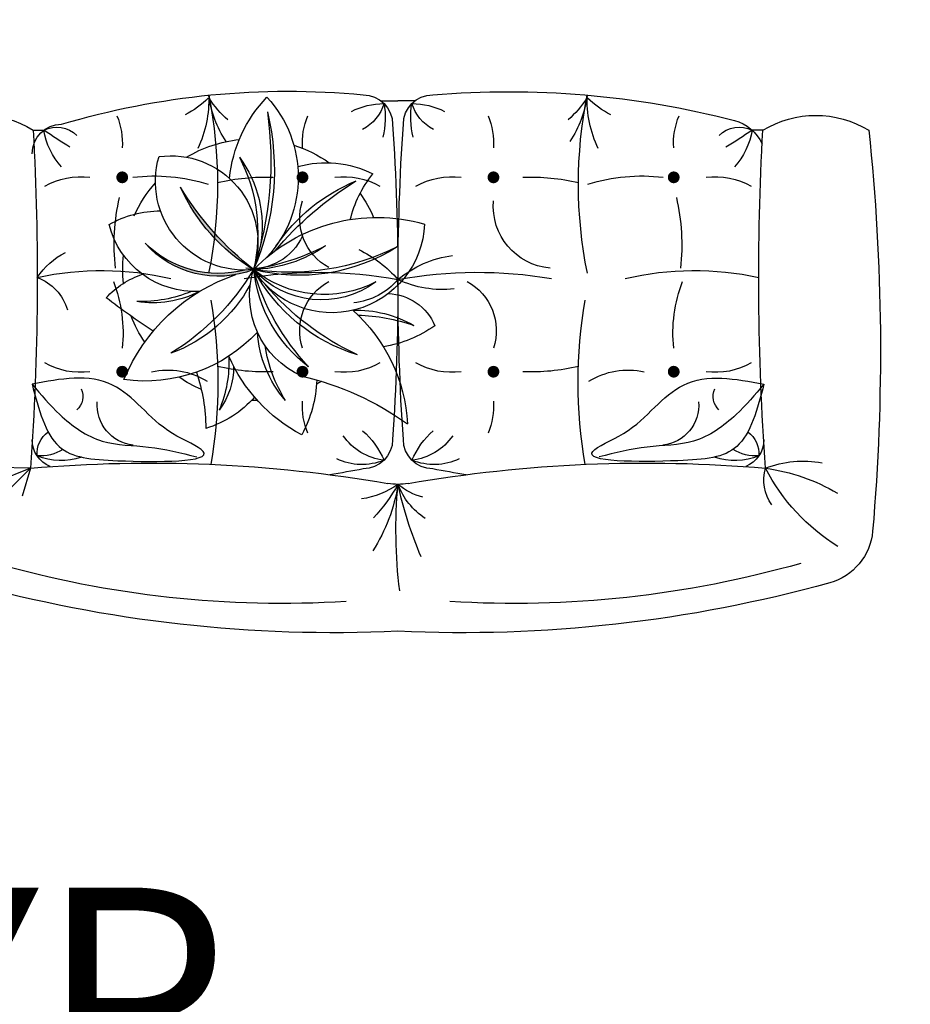
# Model space of a CAD drawing. Units: inches. Extents: x 844 to 2234, y 346 to 1084.
# Tile 5 of 93: x 1112 to 1136, y 653 to 680. Entities that reach past the tile are written whole.
import ezdxf

# ---------------------------------------------------------------- set-up
doc = ezdxf.new("R2010")
doc.units = ezdxf.units.IN
doc.header["$MEASUREMENT"] = 0
doc.layers.add('A-ANNO-DIMS', color=2, linetype='Continuous', lineweight=18)
doc.layers.add('furniture', color=8, linetype='Continuous', lineweight=18)
for name, color, linetype in [('RA-AP-01$0$FURN', 3, 'Continuous'), ('RA-AP-02$0$FLPT', 30, 'Continuous'), ('ROOM-NO', 3, 'Continuous')]:
    doc.layers.add(name, color=color, linetype=linetype)
doc.styles.get("Standard").update_dxf_attribs({"font": 'arial.ttf'})
doc.dimstyles.get("Standard").update_dxf_attribs({"dimtxt": 6, "dimasz": 3, "dimexe": 0.18, "dimexo": 0.0625, "dimgap": 0.09, "dimtad": 0, "dimtih": 1, "dimtoh": 1, "dimdec": 1, "dimzin": 0, "dimdsep": 46, "dimlunit": 3, "dimtxsty": 'Standard', "dimblk": 'ARCHTICK', "dimcen": 0.09, "dimadec": 0, "dimazin": 0, "dimtfac": 1, "dimtdec": 1, "dimtofl": 0, "dimtmove": 0, "dimatfit": 3, "dimfxl": 1, "dimtolj": 1, "dimtzin": 0, "dimarcsym": 0})

# ---------------------------------------------------------------- blocks, each defined once
blk = doc.blocks.new('A$C6E322C05')
at = {"layer": 'RA-AP-01$0$FURN'}
for p, q in [((6.391873508750865, -6.482044957760267), (6.516651486950081, -6.357266979564481)), ((6.391873508750865, -6.482044957760271), (6.43343929223883, -6.37746472106399)), ((6.391873508750866, -6.48204495776027), (6.390422568951521, -6.415535276369585)), ((6.391873508750865, -6.482044957760271), (6.439305270696451, -6.46824831830364)), ((5.817206456966433, -6.486712009544905), (5.817206456965108, -6.505053364959449)), ((5.767206456949363, -7.077520703653457), (5.767206456948565, -7.10671200954539)), ((5.767206456949363, -7.135903315437323), (5.767206456948565, -7.10671200954539)), ((5.817206456966433, -7.726712009545875), (5.817206456965108, -7.70837065413133))]:
    blk.add_line(p, q, dxfattribs=at)
at = {"layer": 'RA-AP-01$0$FURN', "const_width": 0.01}
for points in [[(5.902459393885763, -6.638129816788149, 1), (5.892459393885761, -6.638129816788122, 1)], [(6.222844373610339, -6.638129816788595, -1), (6.23284437361034, -6.638129816788595, -1)], [(5.902459393885763, -6.944444251846759, -1), (5.892459393885761, -6.944444251846785, -1)], [(6.222844373610339, -6.944444251846313, 1), (6.23284437361034, -6.944444251846313, 1)], [(5.902459393885763, -7.268979767244021, 1), (5.892459393885761, -7.268979767243994, 1)], [(6.222844373610339, -7.268979767244466, -1), (6.23284437361034, -7.268979767244466, -1)], [(5.902459393885763, -7.575294202302631, -1), (5.892459393885761, -7.575294202302657, -1)], [(6.222844373610339, -7.575294202302185, 1), (6.23284437361034, -7.575294202302185, 1)]]:
    blk.add_lwpolyline(points, format="xyb", close=True, dxfattribs=at)
at = {"layer": 'RA-AP-01$0$FURN'}
for centre, radius, start, end in [((6.192206456970573, -9.839674509409203), 3.552808610866049, 85.0473312316412, 96.0588723756579), ((5.962206456956505, -6.396712009545393), 0.1706604816468166, 148.1725534208377, 211.8274465791593), ((6.490296991311982, -6.399757455669855), 0.1, 15.49949460085664, 85.04733123164101), ((4.33669785707999, -6.99698289606033), 2.33487526667919, 357.3063521928599, 15.49949460085664), ((4.846593614069285, -6.909687157115225), 1.775196618325768, 356.4780136403396, 15.93354743557553), ((5.857266904022845, -6.534972599266733), 0.05, 90.00000000094654, 180), ((6.068281987477935, -2.019830784287151), 4.473931917517753, 266.7828902523826, 274.1477233631118), ((6.367926665937501, -6.54114871013533), 0.0478550828899777, 86.575295631534, 142.6833829238214), ((6.343036863464309, -6.534972599266733), 0.05, 22.58267242460392, 89.99999999905346), ((6.302747869360707, -6.499593011892033), 0.0683206773889159, 326.6729861493449, 5.218395042636973), ((6.274768375315671, -6.53387763124781), 0.1042084262671507, 340.4828318717155, 22.86929393278168), ((8.747044799885572, -6.68548500417652), 2.363941552380466, 175.0630368065897, 189.8434409139549), ((5.860011614985668, -6.526983908613928), 0.0479292786975047, 152.8070868543555, 225.4025460716553), ((5.798239671935704, -6.625433523557484), 0.1218651776285568, 48.0375529564433, 81.0462320954125), ((4.904259194880517, -7.136565421857206), 1.11020813118073, 31.93286085977143, 34.66647731879807), ((6.017778833798976, -6.566879816788349), 0.1214118203512435, 150.1419074485596, 187.691663289156), ((6.134026645419561, -6.595486433826224), 0.1214600988114338, 123.1053299945123, 153.7006015369794), ((6.565877894706778, -6.603111116245941), 0.5100538472773755, 167.6182489359307, 193.3122231353938), ((6.14746341585187, -6.463466129962243), 0.0853281020358404, 200.7831020638199, 253.0462459140071), ((6.107524933697323, -6.566879816788473), 0.1214118203512435, 352.3083367106845, 29.85809255128089), ((7.09459581372041, -6.919286936999045), 1.343470592134322, 163.3777289595395, 185.4806594039327), ((6.269780256940199, -6.54020363968894), 0.0310151388417235, 245.7760318513891, 317.3789451550392), ((6.284290296802319, -6.664490968717984), 0.0689028341546707, 6.419517109091462, 94.46157264568865), ((6.011601695098697, -6.976164478788355), 0.3517162425384579, 83.41248966761121, 103.1674570565571), ((6.162348040003244, -6.395238182300004), 0.2442261434243043, 248.9017070735605, 275.9923925191661), ((5.839565409091811, -6.517091257029312), 0.1212957045587361, 247.3375839744822, 273.7314750942433), ((6.197523316847625, -6.692545952238853), 0.3023568492824586, 173.0944825511667, 197.588060785551), ((6.354517986346992, -6.715077923337803), 0.1295083186917369, 167.9901339202812, 211.3796151021958), ((5.650260521516567, -6.673548227893377), 0.1579426672576338, 315.4052081938554, 333.0844958846701), ((5.765922189292775, -6.593612516654137), 0.1915923630277471, 267.5852697713958, 295.5830728418392), ((5.908792452070163, -6.03459657477793), 0.765467899454341, 258.6273206109321, 281.4174148186357), ((5.73314461686815, -6.969744817001631), 0.1863549309199891, 56.29262493376822, 82.3818003344588), ((5.679375702373212, -6.920075501166131), 0.1579426672576338, 40.38651175517922, 58.06579944599388), ((6.245858341704271, -5.977214432993086), 0.8232838708255751, 260.2449188973366, 279.7550811026635), ((6.245792934290092, -6.879444251846194), 0.3486563571350461, 166.839178360846, 182.4657575311016), ((5.879510833205829, -6.879444251846704), 0.3486563571350461, 357.5342424690579, 13.1608216393135), ((5.959527339947079, -6.859074294904489), 0.0930420630931112, 293.6025128512426, 6.610683813350465), ((6.80739198570858, -6.9716011229856), 0.7485435294774117, 170.3094183042209, 190.3986311369044), ((5.839565409091811, -7.065482811605596), 0.1212957045587361, 86.2685249057567, 112.6624160255178), ((5.967289987028921, -7.035039638983766), 0.0953802309589454, 28.80342840007747, 108.2253060204472), ((6.158013780467433, -7.035039638983501), 0.0953802309589454, 71.7746939797123, 151.196571600082), ((6.285738358404627, -7.065482811604976), 0.1212957045587361, 67.33758397464167, 93.73147509440282), ((5.08702348459791, -6.791287034316994), 1.330927509443381, 348.8964178164725, 351.3771209523497), ((6.017778833798976, -7.015694251846559), 0.1214118203512435, 172.308336710844, 209.8580925514404), ((6.107524933697323, -7.015694251846435), 0.1214118203512435, 330.1419074487191, 7.691663289315497), ((6.286338558013386, -7.045586518350251), 0.0993499474027353, 337.9047121936679, 25.63436525513283), ((5.904234274973987, -7.085727051545815), 0.1323517050571434, 153.8887786398558, 178.8006589660143), ((6.280014948979332, -7.094901076442985), 0.0990996950214925, 6.922564260119504, 55.10883789097723), ((6.211136556040091, -6.947122539501678), 0.212288550941915, 205.9704430982785, 228.7419974602242), ((5.999456242224805, -7.021102361717039), 0.1116589361851176, 309.9425663137084, 354.6905921774272), ((6.304557655687245, -7.024767404076127), 0.1410608784479501, 324.4849629611242, 351.797284145529), ((5.807266904022846, -7.047601469367252), 0.05, 180, 269.9999999990534), ((5.751472800077547, -7.013313769593298), 0.07258027258109, 286.3558526771587, 332.6774804096085), ((6.4323439288987, -6.955317466880212), 0.1385734111998875, 221.2288777133949, 247.0867614897648), ((6.343036863466045, -7.047601469376512), 0.05, 269.9999999989608, 359.9999999989431), ((6.374625390672053, -6.818147225624045), 0.2920141296149301, 278.8152064253152, 302.6921045175205), ((6.285596300104752, -6.865193601455727), 0.2760944594998999, 298.9825510110601, 313.6694461006315), ((5.795585623761384, -6.952739633017071), 0.1323517050571434, 259.6959164764198, 284.6077968025783), ((6.319376003798462, -7.10671200954539), 0.1, 350.1565590860452, 9.843440913955273), ((6.075151883811576, -3.163731520221818), 3.942980489323571, 266.1043400737264, 273.8956599242929), ((6.075151883808545, -11.04969249895812), 3.942980489412734, 86.10434007575122, 93.89565992614118), ((6.213892115887508, -7.225151532818968), 0.1854874288882049, 140.3167953258794, 172.0522897837384), ((6.80739198570858, -7.241822896105179), 0.7485435294774117, 169.6010516837189, 189.690581695779), ((5.911254573522987, -7.182496879996349), 0.1769409696162427, 353.679636560008, 25.3608296845614), ((6.496371549498975, -7.961935855380467), 0.8586827939016008, 83.03755924582121, 95.14445252709366), ((6.375720249476352, -7.220682794696101), 0.1220457486080966, 33.71356548940426, 69.04099283815023), ((6.338324584842819, -7.175279287582296), 0.1061640434993627, 14.36483859718907, 40.23030537468725), ((6.269502792941208, -7.789055933740261), 0.6986094833441214, 67.00911261779231, 77.61200156369726), ((4.336697857080025, -7.216441123030454), 2.334875266679154, 344.5005053991432, 2.69364780714023), ((5.807266904022846, -7.165822549723527), 0.05, 90.00000000094654, 180), ((5.795585623761384, -7.260684386073708), 0.1323517050571434, 75.39220319742172, 100.3040835235802), ((6.343036863466045, -7.165822549714267), 0.05, 1.0568602e-09, 90.00000000103913), ((8.747044799885572, -7.527939014914259), 2.363941552380466, 170.156559086045, 184.9369631934102), ((5.904234274973987, -7.127696967544965), 0.1323517050571434, 181.1993410339857, 206.1112213601442), ((5.751472800077547, -7.200110249497481), 0.07258027258109, 27.32251959039153, 73.64414732284132), ((6.017778833798976, -7.19772976724422), 0.1214118203512435, 150.1419074485596, 187.691663289156), ((6.107524933697323, -7.197729767244345), 0.1214118203512435, 352.3083367106845, 29.85809255128088), ((6.4323439288987, -7.25810655221026), 0.1385734111998875, 112.9132385102352, 138.7711222866051), ((6.280014948979332, -7.118522942647487), 0.0990996950214925, 304.8911621090228, 353.0774357398805), ((6.286338558013386, -7.167837500740221), 0.0993499474027353, 334.3656347448672, 22.09528780633203), ((7.290981934450236, -7.293982589837588), 1.539060359583382, 175.2233567466078, 194.4661216781742), ((5.08702348459791, -7.422136984773786), 1.330927509443381, 8.62287904765033, 11.10358218352746), ((4.846593614069285, -7.303736861975558), 1.775196618325768, 344.0664525644245, 3.521986359660393), ((6.158013780467433, -7.178384380107278), 0.0953802309589454, 208.803428399918, 288.2253060202877), ((5.839565409091811, -7.147941207485184), 0.1212957045587361, 247.3375839744822, 273.7314750942433), ((6.285738358404627, -7.147941207485803), 0.1212957045587361, 266.2685249055972, 292.6624160253583), ((5.946346035540796, -7.374645549675604), 0.1060388135390937, 5.185910074000148, 94.80734315124221), ((6.245792934290092, -7.333979767244585), 0.3486563571350461, 177.5342424688983, 193.160821639154), ((5.879510833205829, -7.333979767244075), 0.3486563571350461, 346.8391783606865, 2.465757530942165), ((5.679375702373212, -7.293348517924648), 0.1579426672576338, 301.9342005540061, 319.6134882448208), ((5.73314461686815, -7.243679202089149), 0.1863549309199891, 277.6181996655412, 303.7073750662318), ((5.908792452070163, -8.17882744431285), 0.765467899454341, 78.58258518136427, 101.3726793890678), ((6.245858341704271, -8.236209586097694), 0.8232838708255751, 80.24491889733653, 99.75508110266345), ((5.765922189292775, -7.619811502436642), 0.1915923630277471, 64.41692715816083, 92.41473022860427), ((5.650260521516567, -7.539875791197403), 0.1579426672576338, 26.91550411532996, 44.59479180614462), ((6.197523316847625, -7.520878066851927), 0.3023568492824586, 162.411939214449, 186.9055174488332), ((6.354517986346992, -7.498346095752976), 0.1295083186917369, 148.6203848978042, 192.0098660797188), ((6.565877894706778, -7.610312902844838), 0.5100538472773755, 166.6877768646062, 192.3817510640693), ((6.284290296802319, -7.548933050372795), 0.0689028341546707, 265.5384273543114, 353.5804828909086), ((5.839565409091811, -7.696332762061468), 0.1212957045587361, 86.26852490575668, 112.6624160255178), ((6.011601695098697, -7.237259540302424), 0.3517162425384579, 256.8325429434429, 276.5875103323888), ((6.162348040003244, -7.818185836790775), 0.2442261434243043, 84.00760748083387, 111.0982929264395), ((6.017778833798976, -7.646544202302431), 0.1214118203512435, 172.308336710844, 209.8580925514404), ((6.107524933697323, -7.646544202302306), 0.1214118203512435, 330.1419074487191, 7.691663289315504), ((6.269780256940199, -7.67322037940184), 0.0310151388417235, 42.62105484496073, 114.2239681486109), ((6.274768375315671, -7.679546387842969), 0.1042084262671507, 337.1307060672183, 19.51716812828453), ((5.860011614985668, -7.686440110476851), 0.0479292786975047, 134.5974539283447, 207.1929131456445), ((4.904259194880517, -7.076858597233573), 1.11020813118073, 325.333522681202, 328.0671391402286), ((5.87316911435942, -7.657653239374848), 0.0753785023123622, 196.0166452769965, 244.1254380939442), ((5.798239671935704, -7.587990495533295), 0.1218651776285568, 278.9537679045876, 311.9624470435567), ((6.302747869360707, -7.713831007198747), 0.0683206773889159, 354.781604957363, 33.32701385065516), ((6.343036863464309, -7.678451419824046), 0.05, 270.0000000009465, 337.4173275753961), ((6.367926665937501, -7.672275308955449), 0.0478550828899777, 217.3166170761785, 273.424704368466), ((5.966706456956126, -7.816712009545387), 0.1744999999876311, 148.9517780040469, 211.0482219959533), ((6.068281987477935, -12.19359323480363), 4.473931917517753, 85.85227663688822, 93.21710974761734), ((6.549562589740832, -7.794613830093475), 0.1698955038956699, 158.1487616198804, 191.122156864055), ((6.412319729336772, -7.798818772412041), 0.0704710051510922, 53.58735038429053, 106.8661365794674), ((6.713110001951175, -7.687961227420911), 0.3241573581843151, 187.6973649013944, 210.7014325157311), ((6.237117433414106, -8.032110101276656), 0.3382138395168437, 31.74362916573515, 62.76966729059727), ((6.49029699131198, -7.813666563420925), 0.1, 274.9526687683584, 344.500505399143), ((6.192206456970577, -4.373749509681577), 3.552808610866049, 263.941127624342, 274.9526687683587)]:
    blk.add_arc(centre, radius, start, end, dxfattribs=at)
for points, knots in [([(6.249068123947751, -6.484897777661085), (6.239897409094627, -6.533353418276971), (6.226611264288107, -6.603553906267942), (6.290696373977354, -6.673990528916563), (6.332121563214334, -6.713363084361603), (6.381789098403072, -6.831232979612737), (6.381738454094183, -6.629656072516828), (6.370771929626907, -6.516634365426866), (6.291185937762818, -6.495880800642047), (6.249068123947751, -6.484897777661087)], [0, 0, 0, 0, 0.1367586589314792, 0.1981301758052368, 0.2677729570689282, 0.3281194902553322, 0.4737578340741565, 0.5765194025309516, 0.6920332287422236, 0.6920332287422236, 0.6920332287422236, 0.6920332287422236]), ([(6.249068123947751, -6.484897777661087), (6.266851662635476, -6.499857019491296), (6.306238891621481, -6.532988956490432), (6.353826300430336, -6.600137645661404), (6.352465874908733, -6.685122080531377), (6.365878290565239, -6.737689715716581), (6.372748706337224, -6.764617117843226)], [0, 0, 0, 0, 0.070018540671015, 0.1550780383534498, 0.2344491945777043, 0.3178048737568289, 0.3178048737568289, 0.3178048737568289, 0.3178048737568289]), ([(6.249068123947751, -7.728526241429694), (6.239897409094627, -7.680070600813808), (6.226611264288107, -7.609870112822835), (6.290696373977354, -7.539433490174218), (6.332121563214334, -7.500060934729178), (6.381789098403072, -7.382191039478041), (6.381738454094183, -7.583767946573952), (6.370771929626907, -7.696789653663914), (6.291185937762818, -7.717543218448732), (6.249068123947751, -7.728526241429692)], [0, 0, 0, 0, 0.1367586589314792, 0.1981301758052368, 0.2677729570689282, 0.3281194902553322, 0.4737578340741565, 0.5765194025309516, 0.6920332287422236, 0.6920332287422236, 0.6920332287422236, 0.6920332287422236]), ([(6.249068123947751, -7.728526241429692), (6.266851662635476, -7.713566999599485), (6.306238891621481, -7.680435062600349), (6.353826300430336, -7.613286373429378), (6.352465874908733, -7.528301938559401), (6.365878290565239, -7.475734303374198), (6.372748706337224, -7.448806901247554)], [0, 0, 0, 0, 0.070018540671015, 0.1550780383534498, 0.2344491945777043, 0.3178048737568289, 0.3178048737568289, 0.3178048737568289, 0.3178048737568289])]:
    blk.add_open_spline(points, degree=3, knots=knots, dxfattribs=at)
blk = doc.blocks.new('A$C78016F37')
at = {"layer": 'RA-AP-02$0$FLPT'}
for points in [[(8.585816203069419, -6.02390819987247, -0.263770389754008), (8.460672408962632, -5.900531828839305, -0.0241291823863587), (8.454072418949808, -5.887595694471202, 2.53684562776e-05), (8.45404743172537, -5.887630207283394, 0.3135010205465867)], [(8.6375288720004, -5.923949758415821, -0.0887687358956854), (8.454121692088984, -5.887527659105068, 7.7903089823e-06), (8.45411401635844, -5.887538255716633, 0.1521261679004899)]]:
    blk.add_hatch(color=256, dxfattribs=at).paths.add_polyline_path(points)
at = {"layer": 'RA-AP-01$0$FURN'}
for centre, radius, start, end in [((8.676215054199671, -5.667660989702041), 0.3125591380039201, 178.1117989109854, 224.6938723266582), ((8.77416640415315, -5.62926868308301), 0.4113013577889528, 183.916601998098, 218.889069239545), ((8.454024671827373, -5.887489670112504), 0.2224048992971994, 84.85146405771819, 96.8968759960221), ((7.926806489084671, -5.648344237112944), 0.5693232143741963, 340.3683676450975, 358.6332230039188), ((8.195746570571197, -5.703566525505195), 0.3030929277970076, 334.410018118324, 8.056842366720524), ((8.454024671827373, -5.887489670112504), 0.2224048992971994, 48.29632106119188, 65.66234443375417), ((8.028579057188336, -5.942548842808446), 0.3176725093823991, 32.12276904396682, 49.65676958807643), ((8.138392155386812, -5.868774225710474), 0.1937166188785145, 28.24647600965292, 60.3482035660113), ((8.485489110864293, -5.735116799889917), 0.1555876039528135, 173.9896977683083, 258.3326220930856), ((8.521327457039675, -5.708924385009453), 0.1908277389198635, 182.9741757068071, 249.3481441545862), ((8.654249619708994, -5.778555799161595), 0.2279399438329033, 175.7401143551485, 208.5487298435666), ((8.841321835932057, -5.738299260526738), 0.4150383977849519, 183.2217031044116, 201.067141094303), ((8.454024671827373, -5.887489670112504), 0.2224048992971994, 359.5998786150253, 24.14255533511359), ((8.442163868805496, -5.589503946884691), 0.2981456377964393, 227.2393731923049, 272.0875214538299), ((8.499731284894388, -5.433816546692462), 0.4559697329776795, 235.2365058162176, 260.2774785796924), ((8.645911592327788, -6.090477518425219), 0.27932894017942, 93.04938662579335, 133.3896949469156), ((8.610008543493892, -6.006599373458567), 0.1961871509349957, 83.84242350983102, 130.6121505715144), ((8.564547574985227, -5.985184712735347), 0.1475114689626245, 22.41040215178937, 138.5254141817128), ((8.454024671827373, -5.887489670112504), 0.2224048992971994, 179.1222698891959, 181.6416201752811), ((8.343226438185093, -5.786283478281637), 0.1500631261941314, 234.481997856841, 317.590554229248), ((8.35533458686642, -5.671200371653297), 0.2372928460263133, 247.4602721701189, 294.3106346998744), ((8.353310301606033, -5.50080131865886), 0.3995888706145134, 257.1400840392136, 284.5985568218482), ((8.820839898988444, -6.089372712149781), 0.4186128907603021, 151.1845644972185, 178.7925181665867), ((8.647592804319403, -5.39327801538501), 0.5307671632505924, 248.6111860886518, 268.9135435570199), ((8.591324349397098, -5.825721750746069), 0.1505539017216363, 204.2218678925879, 316.713948440902), ((8.60427433017431, -5.61130057980146), 0.3144127437625546, 241.4533621372112, 276.0713675084609), ((8.617925276426345, -5.861018191689067), 0.1660245384207697, 189.1745772070899, 258.8487542743241), ((8.650970463531563, -6.036034461900849), 0.252604074752176, 148.7548044074418, 190.1503402437527), ((8.632043935228618, -5.851861780578565), 0.1781487401371014, 195.8547118906642, 254.9602254039967), ((8.27103219642381, -5.762377687346963), 0.1942058542978326, 259.1738264472347, 296.9361074578899), ((8.242487148295718, -5.713440208635033), 0.2398180026482373, 268.1044384936476, 291.9165885710061), ((8.454024671827373, -5.887489670112504), 0.2224048992971994, 324.5751954876287, 341.8360454133948), ((8.643418645519843, -5.97565241718072), 0.1753165964770544, 183.2000241261284, 219.1319783506275), ((8.454024671827373, -5.887489670112504), 0.2224048992971994, 208.6999597596628, 211.2898901048327), ((8.447576280134497, -6.186493140077375), 0.2128537218708566, 117.7922244992203, 143.1680179163233), ((8.391080266506174, -6.106601067273632), 0.1233275614230441, 120.0065551025349, 157.0200898875673), ((8.702436309821351, -5.965526387054176), 0.2293777808440535, 187.970132899875, 211.770006950379), ((8.454024671827373, -5.887489670112504), 0.2224048992971994, 233.8814212202215, 245.0364073377333), ((8.454024671827373, -5.887489670112504), 0.2224048992971994, 294.3332330132876, 306.7022905924929), ((8.454024671827373, -5.887489670112504), 0.2224048992971994, 266.6746775461067, 279.4836973606225)]:
    blk.add_arc(centre, radius, start, end, dxfattribs=at)
at = {"layer": 'RA-AP-02$0$FLPT'}
blk.add_lwpolyline([(8.373681407360612, -5.597603282219753, 0.7334826821515817), (8.454024671827373, -5.887489670112506, 0.2766279680881699), (8.373681407360612, -5.597603282219752, 1.3559471233864)], format="xyb", dxfattribs=at)
for centre, radius, start, end in [((8.307234168263015, -5.560224752275053), 0.1974581866646199, 313.6950443365965, 339.1517930721081), ((8.39717548070647, -5.778250590985688), 0.1754354389711152, 14.56900959352841, 57.37320031926483), ((8.423880035729836, -5.687934118592295), 0.2086915776254087, 175.0742803806306, 201.2122531761669), ((8.228139151249446, -5.75774524127399), 0.0885717136803359, 32.28640253436571, 97.90409188948885), ((8.433135668112254, -6.051756800567661), 0.1760533926534347, 161.4400574260173, 193.8427700955681), ((8.395985399479063, -6.084837299933293), 0.1497734353479364, 343.3485825573843, 11.74756506179821), ((8.41746442128814, -6.364284642428606), 0.3118134108627832, 101.9980156162763, 119.8647524560376), ((8.942045887600607, -5.120169675385827), 1.085029101271162, 243.0359441902965, 248.2214525024466)]:
    blk.add_arc(centre, radius, start, end, dxfattribs=at)
at = {"layer": 'ROOM-NO'}
for centre, radius, start, end in [((8.65235909715731, -5.915275987506324), 0.2002713751519826, 77.61332513631854, 163.1649854687259), ((8.46944987509335, -5.65497750757116), 0.2349499976215632, 306.2836330402241, 344.0182681768919), ((8.897731643814414, -6.279909663508004), 0.5923422390868573, 112.2662452820337, 138.5100534847894), ((8.794175340646271, -6.133856003178959), 0.4198977696908007, 106.7322927724504, 144.0984247900076), ((8.22288024947718, -6.040653787747125), 0.2772850355038946, 71.89678357893693, 117.3860017964977), ((7.898132843717886, -6.242790504972724), 0.48979813475044, 43.05187184217114, 66.25811984072557), ((8.347851773195234, -6.064576052783105), 0.2064758371609359, 122.2147792747386, 149.2270256684313), ((8.154124515379644, -5.981454547332234), 0.314276155615234, 322.6594768637323, 11.71644421186061), ((8.609526443069848, -6.010438452646774), 0.261483616160276, 163.3494523104177, 218.1824089018609), ((8.3154997513214, -5.724318991124441), 0.2758350084868725, 238.2734303421065, 276.8355613505966), ((8.468611314717652, -6.062483436674201), 0.1756006505860901, 0.6277371554985871, 30.43990742705027), ((8.602078464955955, -5.915823919619132), 0.1507406891149966, 207.5045866236536, 286.2267783265413)]:
    blk.add_arc(centre, radius, start, end, dxfattribs=at)
blk = doc.blocks.new('A$C5D2F253E')
at = {"layer": 'RA-AP-01$0$FURN', "xscale": -1}
blk.add_blockref('A$C6E322C05', (4.620200485489021, 7.961130550668883), dxfattribs=at)
at = {"layer": 'RA-AP-02$0$FLPT', "xscale": -1, "rotation": 210.3787734063952}
blk.add_blockref('A$C78016F37', (-5.749960471669055, -8.254610923396115), dxfattribs=at)
blk = doc.blocks.new('_ArchTick')
at = {"color": 0, "linetype": 'ByBlock', "const_width": 0.15}
blk.add_lwpolyline([(-0.5, -0.5), (0.5, 0.5)], dxfattribs=at)
blk = doc.blocks.new('*D107')
at = {"layer": 'A-ANNO-DIMS', "color": 0, "lineweight": -2, "transparency": 16777216}
for p, q in [((983.441711364941, 646.5161314192717), (983.441711364941, 653.8336314192717)), ((983.441711364941, 653.6536314192717), (1031.441711364941, 653.6536314192717)), ((1031.441711364941, 646.5161314192717), (1031.441711364941, 653.8336314192717)), ((1031.441711364941, 653.6536314192717), (1034.441711364941, 653.6536314192717))]:
    blk.add_line(p, q, dxfattribs=at)
at = {"layer": 'Defpoints', "color": 0, "transparency": 16777216}
for p in [(1031.441711364941, 653.6536314192717), (983.441711364941, 646.4536314192717), (1031.441711364941, 646.4536314192717)]:
    blk.add_point(p, dxfattribs=at)
at = {"layer": 'A-ANNO-DIMS', "color": 0, "lineweight": -2, "transparency": 16777216, "xscale": 3, "yscale": 3, "zscale": 3, "rotation": 180}
blk.add_blockref('_ArchTick', (983.441711364941, 653.6536314192717), dxfattribs=at)
at = {"layer": 'A-ANNO-DIMS', "color": 0, "lineweight": -2, "transparency": 16777216, "xscale": 3, "yscale": 3, "zscale": 3}
blk.add_blockref('_ArchTick', (1031.441711364941, 653.6536314192717), dxfattribs=at)
at = {"layer": 'A-ANNO-DIMS', "color": 0, "transparency": 16777216, "insert": (1078.786827326742, 653.6536314192717), "char_height": 6, "attachment_point": 5}
blk.add_mtext('\\A1;WARDROBE 4\'-0" TYP.', dxfattribs=at)
blk = doc.blocks.new('*D144')
at = {"layer": 'A-ANNO-DIMS', "color": 0, "lineweight": -2, "transparency": 16777216}
for p, q in [((1096.615948, 439.3732739999999), (1096.615948, 1074.743301)), ((1143.115948, 492.373274), (1143.115948, 1074.743301)), ((1096.615948, 1074.563301), (1102.481950728513, 1074.563301)), ((1143.115948, 1074.563301), (1137.249945271487, 1074.563301))]:
    blk.add_line(p, q, dxfattribs=at)
at = {"layer": 'Defpoints', "color": 0, "transparency": 16777216}
for p in [(1143.115948, 1074.563301), (1143.115948, 492.3107739999999), (1096.615948, 439.3107739999999)]:
    blk.add_point(p, dxfattribs=at)
at = {"layer": 'A-ANNO-DIMS', "color": 0, "lineweight": -2, "transparency": 16777216, "xscale": 3, "yscale": 3, "zscale": 3, "rotation": 180}
blk.add_blockref('_ArchTick', (1096.615948, 1074.563301), dxfattribs=at)
at = {"layer": 'A-ANNO-DIMS', "color": 0, "lineweight": -2, "transparency": 16777216, "xscale": 3, "yscale": 3, "zscale": 3}
blk.add_blockref('_ArchTick', (1143.115948, 1074.563301), dxfattribs=at)
at = {"layer": 'A-ANNO-DIMS', "color": 0, "transparency": 16777216, "insert": (1119.865948, 1074.563301), "char_height": 6, "attachment_point": 5}
blk.add_mtext('\\A1;3\'-10 1/2"', dxfattribs=at)

msp = doc.modelspace()

# ---------------------------------------------------------------- block references
at = {"layer": 'furniture', "xscale": 15.94108302203742, "yscale": 15.94108302203742, "zscale": 15.94108302203742, "rotation": 90}
msp.add_blockref('A$C5D2F253E', (1136.147844094663, 696.2584716700112), dxfattribs=at)

# ---------------------------------------------------------------- dimensions: what is measured, and where the dimension line sits
at = {"layer": 'A-ANNO-DIMS'}
dim = msp.add_linear_dim(base=(1143.115948, 1074.563301), p1=(1096.615948, 439.3107739999999), p2=(1143.115948, 492.3107739999999), dimstyle='Standard', override={"dimdec": 1, "dimlfac": 1, "dimrnd": 0, "dimzin": 1, "dimdsep": 46, "dimlunit": 4, "dimfrac": 2}, dxfattribs=at)
dim.commit()
dim.dimension.update_dxf_attribs({"geometry": '*D144', "text_midpoint": (1119.865948, 1074.563301)})
dim = msp.add_linear_dim(base=(1031.441711364941, 653.6536314192717), p1=(983.441711364941, 646.4536314192717), p2=(1031.441711364941, 646.4536314192717), text='WARDROBE <> TYP.', dimstyle='Standard', override={"dimdec": 1, "dimlfac": 1, "dimrnd": 0, "dimzin": 1, "dimdsep": 46, "dimlunit": 4, "dimfrac": 2}, dxfattribs=at)
dim.commit()
dim.dimension.update_dxf_attribs({"geometry": '*D107', "text_midpoint": (1078.786827326742, 653.6536314192717)})

doc.saveas('drawing.dxf')
